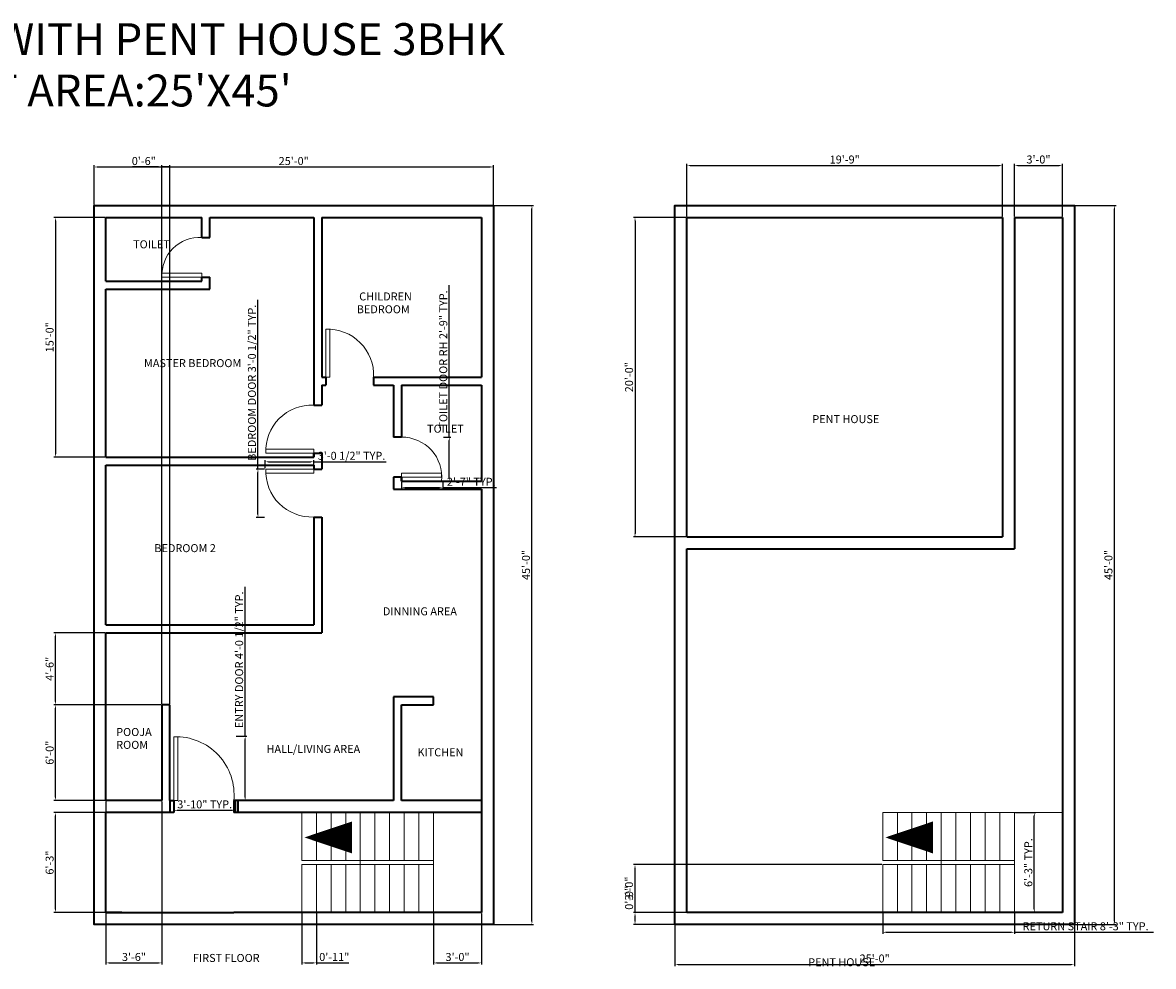
# Model space of a CAD drawing. Units: inches. Extents: x 740 to 2438, y 2555 to 3278.
# Tile 3 of 3: x 1588 to 2438, y 2570 to 3278. Entities that reach past the tile are written whole.
import ezdxf

# ---------------------------------------------------------------- set-up
doc = ezdxf.new("R2010")
doc.units = ezdxf.units.IN
doc.linetypes.add('ACAD_ISO02W100', pattern=[15, 12, -3])
for name, color, linetype, lineweight in [('A-ANNO-DIMS', 2, 'Continuous', 18), ('A-ANNO-TEXT', 7, 'Continuous', 18), ('A-AREA-IDEN', 7, 'Continuous', 18), ('A-DOOR', 3, 'Continuous', 18), ('A-FLOR-STRS', 7, 'Continuous', 18), ('A-FLOR-STRS-PATH', 2, 'ACAD_ISO02W100', 13), ('A-WALL', 7, 'Continuous', 35)]:
    doc.layers.add(name, color=color, linetype=linetype, lineweight=lineweight)
doc.styles.get("Standard").update_dxf_attribs({"font": 'arial.ttf'})
doc.dimstyles.new('ISO-25', dxfattribs={"dimtxt": 6, "dimasz": 2.5, "dimexe": 1.25, "dimexo": 0.625, "dimtad": 1, "dimdec": 1, "dimlunit": 3, "dimtxsty": 'Standard', "dimcen": 2.5, "dimadec": 0, "dimazin": 0, "dimtfac": 1, "dimtdec": 1, "dimtmove": 0, "dimatfit": 3, "dimfxl": 1, "dimarcsym": 0})

# ---------------------------------------------------------------- blocks, each defined once
blk = doc.blocks.new('DOOR-PLAN-48')
blk.add_lwpolyline([(0, 0), (3, 0), (3, 48), (0, 48)], close=True)
blk.add_arc((1.5, 4.3125), 43.7132, 354.3383149, 91.9664646)
blk = doc.blocks.new('DOOR-PLAN-36')
blk.add_lwpolyline([(36, 36), (0, 36), (0, 33), (36, 33)], close=True)
blk.add_arc((34.5, 34.5), 34.53, 177.51045, 272.48955)
blk = doc.blocks.new('DOOR-PLAN-30-L')
blk.add_lwpolyline([(30, 0), (0, 0), (0, 3), (30, 3)], close=True)
blk.add_arc((28.5, 1.5), 28.54, 86.98721, 183.01279)
blk = doc.blocks.new('DOOR-PLAN-30-R')
blk.add_lwpolyline([(0, 3), (30, 3), (30, 6), (0, 6)], close=True)
blk.add_arc((0.15, 3), 30, 354.2609, 90.28648)
blk = doc.blocks.new('STAIR-PLAN-RETURN')
for p, q in [((0, 75), (0, 39)), ((11, 75), (11, 39)), ((22, 75), (22, 39)), ((33, 75), (33, 39)), ((44, 75), (44, 0)), ((55, 75), (55, 39)), ((66, 75), (66, 39)), ((77, 75), (77, 39)), ((88, 75), (88, 39)), ((99, 75), (99, 0)), ((0, 39), (99, 39)), ((0, 36), (99, 36)), ((0, 36), (0, 0)), ((11, 36), (11, 0)), ((22, 36), (22, 0)), ((33, 36), (33, 0)), ((55, 36), (55, 0)), ((66, 36), (66, 0)), ((77, 36), (77, 0)), ((88, 36), (88, 0))]:
    blk.add_line(p, q)
blk = doc.blocks.new('STAIR-PATH-RETURN')
for points in [[(15.6, 0, 0, 0, 0), (114.75, 0, 0, 0, 0), (114.75, 41.58, 0, 0, 0), (35.71, 41.58, 96, 0, 0)], [(35.71, 41.58, 24, 0, 0), (0, 41.58, 0, 0, 0)]]:
    blk.add_lwpolyline(points, format="xyseb")
blk = doc.blocks.new('*D22')
at = {"layer": 'A-ANNO-DIMS', "color": 0, "lineweight": -2, "transparency": 16777216}
for p, q in [((2234.34, 2609.59), (2234.34, 2594.11)), ((2333.34, 2609.59), (2333.34, 2594.11)), ((2236.84, 2595.36), (2330.84, 2595.36)), ((2333.34, 2595.36), (2437.62, 2595.36))]:
    blk.add_line(p, q, dxfattribs=at)
at = {"layer": 'A-ANNO-DIMS', "color": 0, "transparency": 16777216}
for points in [[(2236.84, 2595.78), (2236.84, 2594.95), (2234.34, 2595.36)], [(2330.84, 2595.78), (2330.84, 2594.95), (2333.34, 2595.36)]]:
    blk.add_solid(points, dxfattribs=at)
at = {"layer": 'Defpoints', "color": 0, "transparency": 16777216}
for p in [(2234.34, 2610.21), (2333.34, 2610.21), (2333.34, 2595.36)]:
    blk.add_point(p, dxfattribs=at)
at = {"layer": 'A-ANNO-DIMS', "color": 0, "transparency": 16777216, "insert": (2386.73, 2599.09), "char_height": 6, "attachment_point": 5}
blk.add_mtext('RETURN STAIR 8\'-3" TYP.', dxfattribs=at)
blk = doc.blocks.new('*D23')
at = {"layer": 'A-ANNO-DIMS', "color": 0, "lineweight": -2, "transparency": 16777216}
for p, q in [((2333.97, 2685.21), (2349.44, 2685.21)), ((2348.19, 2612.71), (2348.19, 2682.71)), ((2333.97, 2610.21), (2349.44, 2610.21))]:
    blk.add_line(p, q, dxfattribs=at)
at = {"layer": 'A-ANNO-DIMS', "color": 0, "transparency": 16777216}
for points in [[(2347.78, 2682.71), (2348.61, 2682.71), (2348.19, 2685.21)], [(2347.78, 2612.71), (2348.61, 2612.71), (2348.19, 2610.21)]]:
    blk.add_solid(points, dxfattribs=at)
at = {"layer": 'Defpoints', "color": 0, "transparency": 16777216}
for p in [(2333.34, 2685.21), (2348.19, 2685.21), (2333.34, 2610.21)]:
    blk.add_point(p, dxfattribs=at)
at = {"layer": 'A-ANNO-DIMS', "color": 0, "transparency": 16777216, "insert": (2344.5, 2647.71), "char_height": 6, "attachment_point": 5, "rotation": 90}
blk.add_mtext('6\'-3" TYP.', dxfattribs=at)
blk = doc.blocks.new('*D24')
at = {"layer": 'A-ANNO-DIMS', "color": 0, "lineweight": -2, "transparency": 16777216}
for p, q in [((1765.18, 2943.21), (1765.18, 3070.36)), ((1770.02, 2943.21), (1763.93, 2943.21)), ((1765.18, 2909.29), (1765.18, 2940.71)), ((1770.02, 2906.79), (1763.93, 2906.79))]:
    blk.add_line(p, q, dxfattribs=at)
at = {"layer": 'A-ANNO-DIMS', "color": 0, "transparency": 16777216}
for points in [[(1764.77, 2940.71), (1765.6, 2940.71), (1765.18, 2943.21)], [(1764.77, 2909.29), (1765.6, 2909.29), (1765.18, 2906.79)]]:
    blk.add_solid(points, dxfattribs=at)
at = {"layer": 'Defpoints', "color": 0, "transparency": 16777216}
for p in [(1765.18, 2943.21), (1770.65, 2943.21), (1770.65, 2906.79)]:
    blk.add_point(p, dxfattribs=at)
at = {"layer": 'A-ANNO-DIMS', "color": 0, "transparency": 16777216, "insert": (1761.45, 3008.04), "char_height": 6, "attachment_point": 5, "rotation": 90}
blk.add_mtext('BEDROOM DOOR 3\'-0 1/2" TYP.', dxfattribs=at)
blk = doc.blocks.new('*D25')
at = {"layer": 'A-ANNO-DIMS', "color": 0, "lineweight": -2, "transparency": 16777216}
for p, q in [((1770.65, 2943.84), (1770.65, 2949.93)), ((1773.15, 2948.68), (1804.57, 2948.68)), ((1807.07, 2943.84), (1807.07, 2949.93)), ((1807.07, 2948.68), (1861.37, 2948.68))]:
    blk.add_line(p, q, dxfattribs=at)
at = {"layer": 'A-ANNO-DIMS', "color": 0, "transparency": 16777216}
for points in [[(1773.15, 2949.09), (1773.15, 2948.26), (1770.65, 2948.68)], [(1804.57, 2949.09), (1804.57, 2948.26), (1807.07, 2948.68)]]:
    blk.add_solid(points, dxfattribs=at)
at = {"layer": 'Defpoints', "color": 0, "transparency": 16777216}
for p in [(1807.07, 2948.68), (1770.65, 2943.21), (1807.07, 2943.21)]:
    blk.add_point(p, dxfattribs=at)
at = {"layer": 'A-ANNO-DIMS', "color": 0, "transparency": 16777216, "insert": (1835.47, 2952.41), "char_height": 6, "attachment_point": 5}
blk.add_mtext('3\'-0 1/2" TYP.', dxfattribs=at)
blk = doc.blocks.new('*D26')
at = {"layer": 'A-ANNO-DIMS', "color": 0, "lineweight": -2, "transparency": 16777216}
for p, q in [((1755.58, 2742.65), (1755.58, 2854.85)), ((1748.94, 2742.65), (1756.83, 2742.65)), ((1755.58, 2696.71), (1755.58, 2740.15)), ((1748.94, 2694.21), (1756.83, 2694.21))]:
    blk.add_line(p, q, dxfattribs=at)
at = {"layer": 'A-ANNO-DIMS', "color": 0, "transparency": 16777216}
for points in [[(1755.16, 2740.15), (1755.99, 2740.15), (1755.58, 2742.65)], [(1755.16, 2696.71), (1755.99, 2696.71), (1755.58, 2694.21)]]:
    blk.add_solid(points, dxfattribs=at)
at = {"layer": 'Defpoints', "color": 0, "transparency": 16777216}
for p in [(1748.31, 2742.65), (1755.58, 2742.65), (1748.31, 2694.21)]:
    blk.add_point(p, dxfattribs=at)
at = {"layer": 'A-ANNO-DIMS', "color": 0, "transparency": 16777216, "insert": (1751.85, 2800), "char_height": 6, "attachment_point": 5, "rotation": 90}
blk.add_mtext('ENTRY DOOR 4\'-0 1/2" TYP.', dxfattribs=at)
blk = doc.blocks.new('*D27')
at = {"layer": 'A-ANNO-DIMS', "color": 0, "lineweight": -2, "transparency": 16777216}
for p, q in [((1702.07, 2693.59), (1702.07, 2685.7)), ((1748.31, 2693.59), (1748.31, 2685.7)), ((1704.57, 2686.95), (1745.81, 2686.95))]:
    blk.add_line(p, q, dxfattribs=at)
at = {"layer": 'A-ANNO-DIMS', "color": 0, "transparency": 16777216}
for points in [[(1704.57, 2687.36), (1704.57, 2686.53), (1702.07, 2686.95)], [(1745.81, 2687.36), (1745.81, 2686.53), (1748.31, 2686.95)]]:
    blk.add_solid(points, dxfattribs=at)
at = {"layer": 'Defpoints', "color": 0, "transparency": 16777216}
for p in [(1702.07, 2694.21), (1748.31, 2694.21), (1748.31, 2686.95)]:
    blk.add_point(p, dxfattribs=at)
at = {"layer": 'A-ANNO-DIMS', "color": 0, "transparency": 16777216, "insert": (1725.19, 2690.64), "char_height": 6, "attachment_point": 5}
blk.add_mtext('3\'-10" TYP.', dxfattribs=at)
blk = doc.blocks.new('*D30')
at = {"layer": 'A-ANNO-DIMS', "color": 0, "lineweight": -2, "transparency": 16777216}
for p, q in [((1908.87, 2967.26), (1908.87, 3081.31)), ((1904.54, 2967.26), (1910.12, 2967.26)), ((1908.87, 2936.71), (1908.87, 2964.76)), ((1904.54, 2934.21), (1910.12, 2934.21))]:
    blk.add_line(p, q, dxfattribs=at)
at = {"layer": 'A-ANNO-DIMS', "color": 0, "transparency": 16777216}
for points in [[(1908.46, 2964.76), (1909.29, 2964.76), (1908.87, 2967.26)], [(1908.46, 2936.71), (1909.29, 2936.71), (1908.87, 2934.21)]]:
    blk.add_solid(points, dxfattribs=at)
at = {"layer": 'Defpoints', "color": 0, "transparency": 16777216}
for p in [(1903.92, 2967.26), (1908.87, 2967.26), (1903.92, 2934.21)]:
    blk.add_point(p, dxfattribs=at)
at = {"layer": 'A-ANNO-DIMS', "color": 0, "transparency": 16777216, "insert": (1905.15, 3025.53), "char_height": 6, "attachment_point": 5, "rotation": 90}
blk.add_mtext('TOILET DOOR RH 2\'-9" TYP.', dxfattribs=at)
blk = doc.blocks.new('*D31')
at = {"layer": 'A-ANNO-DIMS', "color": 0, "lineweight": -2, "transparency": 16777216}
for p, q in [((1873.07, 2933.59), (1873.07, 2928.01)), ((1903.92, 2933.59), (1903.92, 2928.01)), ((1875.57, 2929.26), (1901.42, 2929.26)), ((1903.92, 2929.26), (1944.34, 2929.26))]:
    blk.add_line(p, q, dxfattribs=at)
at = {"layer": 'A-ANNO-DIMS', "color": 0, "transparency": 16777216}
for points in [[(1875.57, 2929.67), (1875.57, 2928.84), (1873.07, 2929.26)], [(1901.42, 2929.67), (1901.42, 2928.84), (1903.92, 2929.26)]]:
    blk.add_solid(points, dxfattribs=at)
at = {"layer": 'Defpoints', "color": 0, "transparency": 16777216}
for p in [(1873.07, 2934.21), (1903.92, 2934.21), (1903.92, 2929.26)]:
    blk.add_point(p, dxfattribs=at)
at = {"layer": 'A-ANNO-DIMS', "color": 0, "transparency": 16777216, "insert": (1925.38, 2932.9), "char_height": 6, "attachment_point": 5}
blk.add_mtext('2\'-7" TYP.', dxfattribs=at)
blk = doc.blocks.new('*D34')
at = {"layer": 'A-ANNO-DIMS', "color": 0, "lineweight": -2, "transparency": 16777216}
for p, q in [((1642.07, 3141.84), (1642.07, 3171.31)), ((1644.57, 3170.06), (1939.57, 3170.06)), ((1942.07, 3141.84), (1942.07, 3171.31))]:
    blk.add_line(p, q, dxfattribs=at)
at = {"layer": 'A-ANNO-DIMS', "color": 0, "transparency": 16777216}
for points in [[(1644.57, 3170.48), (1644.57, 3169.65), (1642.07, 3170.06)], [(1939.57, 3170.48), (1939.57, 3169.65), (1942.07, 3170.06)]]:
    blk.add_solid(points, dxfattribs=at)
at = {"layer": 'Defpoints', "color": 0, "transparency": 16777216}
for p in [(1942.07, 3170.06), (1642.07, 3141.21), (1942.07, 3141.21)]:
    blk.add_point(p, dxfattribs=at)
at = {"layer": 'A-ANNO-DIMS', "color": 0, "transparency": 16777216, "insert": (1792.07, 3173.75), "char_height": 6, "attachment_point": 5}
blk.add_mtext('25\'-0"', dxfattribs=at)
blk = doc.blocks.new('*D35')
at = {"layer": 'A-ANNO-DIMS', "color": 0, "lineweight": -2, "transparency": 16777216}
for p, q in [((1942.69, 3141.21), (1972.17, 3141.21)), ((1970.92, 2603.71), (1970.92, 3138.71)), ((1942.69, 2601.21), (1972.17, 2601.21))]:
    blk.add_line(p, q, dxfattribs=at)
at = {"layer": 'A-ANNO-DIMS', "color": 0, "transparency": 16777216}
for points in [[(1970.5, 3138.71), (1971.33, 3138.71), (1970.92, 3141.21)], [(1970.5, 2603.71), (1971.33, 2603.71), (1970.92, 2601.21)]]:
    blk.add_solid(points, dxfattribs=at)
at = {"layer": 'Defpoints', "color": 0, "transparency": 16777216}
for p in [(1942.07, 3141.21), (1970.92, 3141.21), (1942.07, 2601.21)]:
    blk.add_point(p, dxfattribs=at)
at = {"layer": 'A-ANNO-DIMS', "color": 0, "transparency": 16777216, "insert": (1967.23, 2871.21), "char_height": 6, "attachment_point": 5, "rotation": 90}
blk.add_mtext('45\'-0"', dxfattribs=at)
blk = doc.blocks.new('*D36')
at = {"layer": 'A-ANNO-DIMS', "color": 0, "lineweight": -2, "transparency": 16777216}
for p, q in [((2078.34, 2600.59), (2078.34, 2569.96)), ((2378.34, 2600.59), (2378.34, 2569.96)), ((2080.84, 2571.21), (2375.84, 2571.21))]:
    blk.add_line(p, q, dxfattribs=at)
at = {"layer": 'A-ANNO-DIMS', "color": 0, "transparency": 16777216}
for points in [[(2080.84, 2571.63), (2080.84, 2570.8), (2078.34, 2571.21)], [(2375.84, 2571.63), (2375.84, 2570.8), (2378.34, 2571.21)]]:
    blk.add_solid(points, dxfattribs=at)
at = {"layer": 'Defpoints', "color": 0, "transparency": 16777216}
for p in [(2078.34, 2601.21), (2378.34, 2601.21), (2378.34, 2571.21)]:
    blk.add_point(p, dxfattribs=at)
at = {"layer": 'A-ANNO-DIMS', "color": 0, "transparency": 16777216, "insert": (2228.34, 2574.9), "char_height": 6, "attachment_point": 5}
blk.add_mtext('25\'-0"', dxfattribs=at)
blk = doc.blocks.new('*D37')
at = {"layer": 'A-ANNO-DIMS', "color": 0, "lineweight": -2, "transparency": 16777216}
for p, q in [((2378.97, 3141.21), (2409.59, 3141.21)), ((2408.34, 2603.71), (2408.34, 3138.71)), ((2378.97, 2601.21), (2409.59, 2601.21))]:
    blk.add_line(p, q, dxfattribs=at)
at = {"layer": 'A-ANNO-DIMS', "color": 0, "transparency": 16777216}
for points in [[(2407.93, 3138.71), (2408.76, 3138.71), (2408.34, 3141.21)], [(2407.93, 2603.71), (2408.76, 2603.71), (2408.34, 2601.21)]]:
    blk.add_solid(points, dxfattribs=at)
at = {"layer": 'Defpoints', "color": 0, "transparency": 16777216}
for p in [(2378.34, 3141.21), (2408.34, 3141.21), (2378.34, 2601.21)]:
    blk.add_point(p, dxfattribs=at)
at = {"layer": 'A-ANNO-DIMS', "color": 0, "transparency": 16777216, "insert": (2404.66, 2871.21), "char_height": 6, "attachment_point": 5, "rotation": 90}
blk.add_mtext('45\'-0"', dxfattribs=at)
blk = doc.blocks.new('*D38')
at = {"layer": 'A-ANNO-DIMS', "color": 0, "lineweight": -2, "transparency": 16777216}
for p, q in [((2087.34, 3132.84), (2087.34, 3172.46)), ((2089.84, 3171.21), (2321.84, 3171.21)), ((2324.34, 3132.84), (2324.34, 3172.46))]:
    blk.add_line(p, q, dxfattribs=at)
at = {"layer": 'A-ANNO-DIMS', "color": 0, "transparency": 16777216}
for points in [[(2089.84, 3171.63), (2089.84, 3170.8), (2087.34, 3171.21)], [(2321.84, 3171.63), (2321.84, 3170.8), (2324.34, 3171.21)]]:
    blk.add_solid(points, dxfattribs=at)
at = {"layer": 'Defpoints', "color": 0, "transparency": 16777216}
for p in [(2324.34, 3171.21), (2087.34, 3132.21), (2324.34, 3132.21)]:
    blk.add_point(p, dxfattribs=at)
at = {"layer": 'A-ANNO-DIMS', "color": 0, "transparency": 16777216, "insert": (2205.84, 3174.9), "char_height": 6, "attachment_point": 5}
blk.add_mtext('19\'-9"', dxfattribs=at)
blk = doc.blocks.new('*D39')
at = {"layer": 'A-ANNO-DIMS', "color": 0, "lineweight": -2, "transparency": 16777216}
for p, q in [((2086.72, 3132.21), (2047.09, 3132.21)), ((2048.34, 3129.71), (2048.34, 2894.71)), ((2086.72, 2892.21), (2047.09, 2892.21))]:
    blk.add_line(p, q, dxfattribs=at)
at = {"layer": 'A-ANNO-DIMS', "color": 0, "transparency": 16777216}
for points in [[(2047.93, 3129.71), (2048.76, 3129.71), (2048.34, 3132.21)], [(2047.93, 2894.71), (2048.76, 2894.71), (2048.34, 2892.21)]]:
    blk.add_solid(points, dxfattribs=at)
at = {"layer": 'Defpoints', "color": 0, "transparency": 16777216}
for p in [(2087.34, 3132.21), (2048.34, 2892.21), (2087.34, 2892.21)]:
    blk.add_point(p, dxfattribs=at)
at = {"layer": 'A-ANNO-DIMS', "color": 0, "transparency": 16777216, "insert": (2044.66, 3012.21), "char_height": 6, "attachment_point": 5, "rotation": 90}
blk.add_mtext('20\'-0"', dxfattribs=at)
blk = doc.blocks.new('*D40')
at = {"layer": 'A-ANNO-DIMS', "color": 0, "lineweight": -2, "transparency": 16777216}
for p, q in [((2333.34, 3132.84), (2333.34, 3172.46)), ((2335.84, 3171.21), (2366.84, 3171.21)), ((2369.34, 3132.84), (2369.34, 3172.46))]:
    blk.add_line(p, q, dxfattribs=at)
at = {"layer": 'A-ANNO-DIMS', "color": 0, "transparency": 16777216}
for points in [[(2335.84, 3171.63), (2335.84, 3170.8), (2333.34, 3171.21)], [(2366.84, 3171.63), (2366.84, 3170.8), (2369.34, 3171.21)]]:
    blk.add_solid(points, dxfattribs=at)
at = {"layer": 'Defpoints', "color": 0, "transparency": 16777216}
for p in [(2369.34, 3171.21), (2333.34, 3132.21), (2369.34, 3132.21)]:
    blk.add_point(p, dxfattribs=at)
at = {"layer": 'A-ANNO-DIMS', "color": 0, "transparency": 16777216, "insert": (2351.34, 3174.9), "char_height": 6, "attachment_point": 5}
blk.add_mtext('3\'-0"', dxfattribs=at)
blk = doc.blocks.new('*D41')
at = {"layer": 'A-ANNO-DIMS', "color": 0, "lineweight": -2, "transparency": 16777216}
for p, q in [((2048.34, 2610.21), (2048.34, 2629.91)), ((2086.72, 2610.21), (2047.09, 2610.21)), ((2048.34, 2603.71), (2048.34, 2607.71)), ((2077.72, 2601.21), (2047.09, 2601.21))]:
    blk.add_line(p, q, dxfattribs=at)
at = {"layer": 'A-ANNO-DIMS', "color": 0, "transparency": 16777216}
for points in [[(2047.93, 2607.71), (2048.76, 2607.71), (2048.34, 2610.21)], [(2047.93, 2603.71), (2048.76, 2603.71), (2048.34, 2601.21)]]:
    blk.add_solid(points, dxfattribs=at)
at = {"layer": 'Defpoints', "color": 0, "transparency": 16777216}
for p in [(2048.34, 2610.21), (2087.34, 2610.21), (2078.34, 2601.21)]:
    blk.add_point(p, dxfattribs=at)
at = {"layer": 'A-ANNO-DIMS', "color": 0, "transparency": 16777216, "insert": (2044.66, 2621.31), "char_height": 6, "attachment_point": 5, "rotation": 90}
blk.add_mtext('0\'-9"', dxfattribs=at)
blk = doc.blocks.new('*D42')
at = {"layer": 'A-ANNO-DIMS', "color": 0, "lineweight": -2, "transparency": 16777216}
for p, q in [((2233.72, 2646.21), (2047.09, 2646.21)), ((2048.34, 2612.71), (2048.34, 2643.71)), ((2233.72, 2610.21), (2047.09, 2610.21))]:
    blk.add_line(p, q, dxfattribs=at)
at = {"layer": 'A-ANNO-DIMS', "color": 0, "transparency": 16777216}
for points in [[(2047.93, 2643.71), (2048.76, 2643.71), (2048.34, 2646.21)], [(2047.93, 2612.71), (2048.76, 2612.71), (2048.34, 2610.21)]]:
    blk.add_solid(points, dxfattribs=at)
at = {"layer": 'Defpoints', "color": 0, "transparency": 16777216}
for p in [(2048.34, 2646.21), (2234.34, 2646.21), (2234.34, 2610.21)]:
    blk.add_point(p, dxfattribs=at)
at = {"layer": 'A-ANNO-DIMS', "color": 0, "transparency": 16777216, "insert": (2044.65, 2628.21), "char_height": 6, "attachment_point": 5, "rotation": 90}
blk.add_mtext('3\'-0"', dxfattribs=at)
blk = doc.blocks.new('*D43')
at = {"layer": 'A-ANNO-DIMS', "color": 0, "lineweight": -2, "transparency": 16777216}
for p, q in [((1798.07, 2609.59), (1798.07, 2571.11)), ((1809.07, 2609.59), (1809.07, 2571.11)), ((1800.57, 2572.36), (1806.57, 2572.36)), ((1809.07, 2572.36), (1833.43, 2572.36))]:
    blk.add_line(p, q, dxfattribs=at)
at = {"layer": 'A-ANNO-DIMS', "color": 0, "transparency": 16777216}
for points in [[(1800.57, 2572.78), (1800.57, 2571.95), (1798.07, 2572.36)], [(1806.57, 2572.78), (1806.57, 2571.95), (1809.07, 2572.36)]]:
    blk.add_solid(points, dxfattribs=at)
at = {"layer": 'Defpoints', "color": 0, "transparency": 16777216}
for p in [(1798.07, 2610.21), (1809.07, 2610.21), (1809.07, 2572.36)]:
    blk.add_point(p, dxfattribs=at)
at = {"layer": 'A-ANNO-DIMS', "color": 0, "transparency": 16777216, "insert": (1822.5, 2576.05), "char_height": 6, "attachment_point": 5}
blk.add_mtext('0\'-11"', dxfattribs=at)
blk = doc.blocks.new('*D44')
at = {"layer": 'A-ANNO-DIMS', "color": 0, "lineweight": -2, "transparency": 16777216}
for p, q in [((1897.07, 2609.59), (1897.07, 2571.11)), ((1933.07, 2609.59), (1933.07, 2571.11)), ((1899.57, 2572.36), (1930.57, 2572.36))]:
    blk.add_line(p, q, dxfattribs=at)
at = {"layer": 'A-ANNO-DIMS', "color": 0, "transparency": 16777216}
for points in [[(1899.57, 2572.78), (1899.57, 2571.95), (1897.07, 2572.36)], [(1930.57, 2572.78), (1930.57, 2571.95), (1933.07, 2572.36)]]:
    blk.add_solid(points, dxfattribs=at)
at = {"layer": 'Defpoints', "color": 0, "transparency": 16777216}
for p in [(1897.07, 2610.21), (1933.07, 2610.21), (1933.07, 2572.36)]:
    blk.add_point(p, dxfattribs=at)
at = {"layer": 'A-ANNO-DIMS', "color": 0, "transparency": 16777216, "insert": (1915.07, 2576.05), "char_height": 6, "attachment_point": 5}
blk.add_mtext('3\'-0"', dxfattribs=at)
blk = doc.blocks.new('*D71')
at = {"layer": 'A-ANNO-DIMS', "color": 0, "lineweight": -2, "transparency": 16777216}
for p, q in [((1651.07, 2693.59), (1651.07, 2571.11)), ((1693.07, 2693.59), (1693.07, 2571.11)), ((1653.57, 2572.36), (1690.57, 2572.36))]:
    blk.add_line(p, q, dxfattribs=at)
at = {"layer": 'A-ANNO-DIMS', "color": 0, "transparency": 16777216}
for points in [[(1653.57, 2572.78), (1653.57, 2571.95), (1651.07, 2572.36)], [(1690.57, 2572.78), (1690.57, 2571.95), (1693.07, 2572.36)]]:
    blk.add_solid(points, dxfattribs=at)
at = {"layer": 'Defpoints', "color": 0, "transparency": 16777216}
for p in [(1651.07, 2694.21), (1693.07, 2694.21), (1693.07, 2572.36)]:
    blk.add_point(p, dxfattribs=at)
at = {"layer": 'A-ANNO-DIMS', "color": 0, "transparency": 16777216, "insert": (1672.07, 2576.05), "char_height": 6, "attachment_point": 5}
blk.add_mtext('3\'-6"', dxfattribs=at)
blk = doc.blocks.new('*D72')
at = {"layer": 'A-ANNO-DIMS', "color": 0, "lineweight": -2, "transparency": 16777216}
for p, q in [((1692.44, 2766.21), (1611.97, 2766.21)), ((1613.22, 2696.71), (1613.22, 2763.71)), ((1692.44, 2694.21), (1611.97, 2694.21))]:
    blk.add_line(p, q, dxfattribs=at)
at = {"layer": 'A-ANNO-DIMS', "color": 0, "transparency": 16777216}
for points in [[(1612.8, 2763.71), (1613.63, 2763.71), (1613.22, 2766.21)], [(1612.8, 2696.71), (1613.63, 2696.71), (1613.22, 2694.21)]]:
    blk.add_solid(points, dxfattribs=at)
at = {"layer": 'Defpoints', "color": 0, "transparency": 16777216}
for p in [(1613.22, 2766.21), (1693.07, 2766.21), (1693.07, 2694.21)]:
    blk.add_point(p, dxfattribs=at)
at = {"layer": 'A-ANNO-DIMS', "color": 0, "transparency": 16777216, "insert": (1609.53, 2730.21), "char_height": 6, "attachment_point": 5, "rotation": 90}
blk.add_mtext('6\'-0"', dxfattribs=at)
blk = doc.blocks.new('*D73')
at = {"layer": 'A-ANNO-DIMS', "color": 0, "lineweight": -2, "transparency": 16777216}
for p, q in [((1650.44, 2820.21), (1611.97, 2820.21)), ((1613.22, 2768.71), (1613.22, 2817.71)), ((1692.44, 2766.21), (1611.97, 2766.21))]:
    blk.add_line(p, q, dxfattribs=at)
at = {"layer": 'A-ANNO-DIMS', "color": 0, "transparency": 16777216}
for points in [[(1612.8, 2817.71), (1613.63, 2817.71), (1613.22, 2820.21)], [(1612.8, 2768.71), (1613.63, 2768.71), (1613.22, 2766.21)]]:
    blk.add_solid(points, dxfattribs=at)
at = {"layer": 'Defpoints', "color": 0, "transparency": 16777216}
for p in [(1613.22, 2820.21), (1651.07, 2820.21), (1693.07, 2766.21)]:
    blk.add_point(p, dxfattribs=at)
at = {"layer": 'A-ANNO-DIMS', "color": 0, "transparency": 16777216, "insert": (1609.53, 2793.21), "char_height": 6, "attachment_point": 5, "rotation": 90}
blk.add_mtext('4\'-6"', dxfattribs=at)
blk = doc.blocks.new('*D74')
at = {"layer": 'A-ANNO-DIMS', "color": 0, "lineweight": -2, "transparency": 16777216}
for p, q in [((1650.44, 2685.21), (1611.97, 2685.21)), ((1613.22, 2612.71), (1613.22, 2682.71)), ((1650.44, 2610.21), (1611.97, 2610.21))]:
    blk.add_line(p, q, dxfattribs=at)
at = {"layer": 'A-ANNO-DIMS', "color": 0, "transparency": 16777216}
for points in [[(1612.8, 2682.71), (1613.63, 2682.71), (1613.22, 2685.21)], [(1612.8, 2612.71), (1613.63, 2612.71), (1613.22, 2610.21)]]:
    blk.add_solid(points, dxfattribs=at)
at = {"layer": 'Defpoints', "color": 0, "transparency": 16777216}
for p in [(1613.22, 2685.21), (1651.07, 2685.21), (1651.07, 2610.21)]:
    blk.add_point(p, dxfattribs=at)
at = {"layer": 'A-ANNO-DIMS', "color": 0, "transparency": 16777216, "insert": (1609.53, 2647.71), "char_height": 6, "attachment_point": 5, "rotation": 90}
blk.add_mtext('6\'-3"', dxfattribs=at)
blk = doc.blocks.new('*D75')
at = {"layer": 'A-ANNO-DIMS', "color": 0, "lineweight": -2, "transparency": 16777216}
for p, q in [((1650.44, 3132.21), (1611.97, 3132.21)), ((1613.22, 3129.71), (1613.22, 2954.71)), ((1650.44, 2952.21), (1611.97, 2952.21))]:
    blk.add_line(p, q, dxfattribs=at)
at = {"layer": 'A-ANNO-DIMS', "color": 0, "transparency": 16777216}
for points in [[(1612.8, 3129.71), (1613.63, 3129.71), (1613.22, 3132.21)], [(1612.8, 2954.71), (1613.63, 2954.71), (1613.22, 2952.21)]]:
    blk.add_solid(points, dxfattribs=at)
at = {"layer": 'Defpoints', "color": 0, "transparency": 16777216}
for p in [(1651.07, 3132.21), (1613.22, 2952.21), (1651.07, 2952.21)]:
    blk.add_point(p, dxfattribs=at)
at = {"layer": 'A-ANNO-DIMS', "color": 0, "transparency": 16777216, "insert": (1609.53, 3042.21), "char_height": 6, "attachment_point": 5, "rotation": 90}
blk.add_mtext('15\'-0"', dxfattribs=at)
blk = doc.blocks.new('*D78')
at = {"layer": 'A-ANNO-DIMS', "color": 0, "lineweight": -2, "transparency": 16777216}
for p, q in [((1690.57, 3170.06), (1670.87, 3170.06)), ((1693.07, 2766.84), (1693.07, 3171.31)), ((1699.07, 3170.06), (1693.07, 3170.06)), ((1699.07, 2766.84), (1699.07, 3171.31)), ((1701.57, 3170.06), (1704.07, 3170.06))]:
    blk.add_line(p, q, dxfattribs=at)
at = {"layer": 'A-ANNO-DIMS', "color": 0, "transparency": 16777216}
for points in [[(1690.57, 3170.48), (1690.57, 3169.65), (1693.07, 3170.06)], [(1701.57, 3170.48), (1701.57, 3169.65), (1699.07, 3170.06)]]:
    blk.add_solid(points, dxfattribs=at)
at = {"layer": 'Defpoints', "color": 0, "transparency": 16777216}
for p in [(1693.07, 3170.06), (1693.07, 2766.21), (1699.07, 2766.21)]:
    blk.add_point(p, dxfattribs=at)
at = {"layer": 'A-ANNO-DIMS', "color": 0, "transparency": 16777216, "insert": (1679.47, 3173.75), "char_height": 6, "attachment_point": 5}
blk.add_mtext('0\'-6"', dxfattribs=at)

msp = doc.modelspace()

# ---------------------------------------------------------------- linework, layer by layer
at = {"layer": 'A-FLOR-STRS'}
msp.add_line((2234.34, 2685.21), (2369.34, 2685.21), dxfattribs=at)
at = {"layer": 'A-WALL'}
for p, q in [((1651.07, 3132.21), (1723.07, 3132.21)), ((1651.07, 3084.21), (1651.07, 3132.21)), ((1723.07, 3117.21), (1723.07, 3132.21)), ((1729.07, 3132.21), (1807.07, 3132.21)), ((1729.07, 3117.21), (1729.07, 3132.21)), ((1807.07, 3132.21), (1807.07, 2991.21)), ((1813.07, 3132.21), (1933.07, 3132.21)), ((1813.07, 3132.21), (1813.07, 3012.21)), ((1933.07, 3132.21), (1933.07, 3012.21)), ((2087.34, 3132.21), (2324.34, 3132.21)), ((2087.34, 2892.21), (2087.34, 3132.21)), ((2324.34, 3132.21), (2324.34, 2892.21)), ((2333.34, 3132.21), (2333.34, 2883.21)), ((2333.34, 3132.21), (2369.34, 3132.21)), ((2369.34, 3132.21), (2369.34, 2883.21)), ((1723.07, 3117.21), (1729.07, 3117.21)), ((1651.07, 3084.21), (1723.07, 3084.21)), ((1723.07, 3084.21), (1723.07, 3087.21)), ((1723.07, 3084.21), (1723.07, 3087.21)), ((1723.07, 3087.21), (1729.07, 3087.21)), ((1729.07, 3078.21), (1729.07, 3087.21)), ((1651.07, 3078.21), (1729.07, 3078.21)), ((1651.07, 2952.21), (1651.07, 3078.21)), ((1813.07, 3012.21), (1816.07, 3012.21)), ((1813.07, 3012.21), (1816.07, 3012.21)), ((1813.07, 3006.21), (1816.07, 3006.21)), ((1813.07, 3006.21), (1813.07, 2991.21)), ((1816.07, 3012.21), (1816.07, 3006.21)), ((1852.07, 3012.21), (1933.07, 3012.21)), ((1852.07, 3012.21), (1852.07, 3006.21)), ((1852.07, 3006.21), (1867.07, 3006.21)), ((1867.07, 3006.21), (1867.07, 2967.21)), ((1873.07, 3006.21), (1933.07, 3006.21)), ((1873.07, 3006.21), (1873.07, 2967.21)), ((1933.07, 3006.21), (1933.07, 2934.21)), ((1807.07, 2991.21), (1813.07, 2991.21)), ((1873.07, 2967.21), (1867.07, 2967.21)), ((1807.07, 2955.21), (1807.07, 2952.21)), ((1807.07, 2952.21), (1807.07, 2955.21)), ((1807.07, 2955.21), (1813.07, 2955.21)), ((1813.07, 2955.21), (1813.07, 2943.21)), ((1651.07, 2952.21), (1807.07, 2952.21)), ((1651.07, 2946.21), (1807.07, 2946.21)), ((1651.07, 2826.21), (1651.07, 2946.21)), ((1807.07, 2946.21), (1807.07, 2943.21)), ((1807.07, 2946.21), (1807.07, 2943.21)), ((1807.07, 2943.21), (1813.07, 2943.21)), ((1867.07, 2937.21), (1867.07, 2928.21)), ((1873.07, 2937.21), (1867.07, 2937.21)), ((1873.07, 2937.21), (1873.07, 2934.21)), ((1873.07, 2934.21), (1873.07, 2937.21)), ((1873.07, 2934.21), (1933.07, 2934.21)), ((1867.07, 2928.21), (1933.07, 2928.21)), ((1933.07, 2928.21), (1933.07, 2610.21)), ((1807.07, 2907.21), (1807.07, 2826.21)), ((1807.07, 2907.21), (1813.07, 2907.21)), ((1813.07, 2907.21), (1813.07, 2820.21)), ((2087.34, 2892.21), (2324.34, 2892.21)), ((2087.34, 2610.21), (2087.34, 2883.21)), ((2087.34, 2883.21), (2333.34, 2883.21)), ((2369.34, 2883.21), (2369.34, 2610.21)), ((1651.07, 2826.21), (1807.07, 2826.21)), ((1651.07, 2820.21), (1813.07, 2820.21)), ((1651.07, 2694.21), (1651.07, 2820.21)), ((1897.07, 2772.21), (1867.07, 2772.21)), ((1867.07, 2772.21), (1867.07, 2766.21)), ((1897.07, 2766.21), (1897.07, 2772.21)), ((1699.07, 2766.21), (1693.07, 2766.21)), ((1693.07, 2766.21), (1693.07, 2694.21)), ((1699.07, 2694.21), (1699.07, 2766.21)), ((1867.07, 2766.21), (1867.07, 2694.21)), ((1873.07, 2694.21), (1873.07, 2766.21)), ((1873.07, 2766.21), (1897.07, 2766.21)), ((1693.07, 2694.21), (1651.07, 2694.21)), ((1699.07, 2694.21), (1699.07, 2685.21)), ((1699.07, 2694.21), (1702.07, 2694.21)), ((1702.07, 2694.21), (1702.07, 2685.21)), ((1867.07, 2694.21), (1747.07, 2694.21)), ((1747.07, 2694.21), (1747.07, 2685.21)), ((1750.07, 2694.21), (1750.07, 2685.21)), ((1933.07, 2694.21), (1873.07, 2694.21)), ((1699.07, 2685.21), (1651.07, 2685.21)), ((1651.07, 2610.21), (1651.07, 2685.21)), ((1702.07, 2685.21), (1699.07, 2685.21)), ((1933.07, 2685.21), (1747.07, 2685.21)), ((1663.07, 2610.21), (1651.07, 2610.21)), ((1651.07, 2610.21), (1747.07, 2610.21)), ((1933.07, 2610.21), (1747.07, 2610.21)), ((2369.34, 2610.21), (2087.34, 2610.21))]:
    msp.add_line(p, q, dxfattribs=at)
for points in [[(1747.07, 2601.21), (1642.07, 2601.21), (1642.07, 3141.21), (1942.07, 3141.21), (1942.07, 2601.21), (1747.07, 2601.21)], [(2378.34, 2601.21), (2078.34, 2601.21), (2078.34, 3141.21), (2378.34, 3141.21), (2378.34, 2601.21), (2183.34, 2601.21)]]:
    msp.add_lwpolyline(points, dxfattribs=at)

# ---------------------------------------------------------------- block references
at = {"layer": 'A-DOOR'}
for name, p in [('DOOR-PLAN-30-L', (1693.07, 3087.21)), ('DOOR-PLAN-30-R', (1873.07, 2934.21)), ('DOOR-PLAN-36', (1771.07, 2907.21)), ('DOOR-PLAN-48', (1702.07, 2694.21))]:
    msp.add_blockref(name, p, dxfattribs=at)
at = {"layer": 'A-DOOR', "extrusion": (0, 0, -1), "zscale": -1}
for p, rotation in [((-1852.07, 3048.21), 269.9999999999956), ((-1771.07, 2991.21), 180)]:
    msp.add_blockref('DOOR-PLAN-36', p, dxfattribs=dict(at, rotation=rotation))
at = {"layer": 'A-FLOR-STRS'}
for p in [(1798.07, 2610.21), (2234.34, 2610.21)]:
    msp.add_blockref('STAIR-PLAN-RETURN', p, dxfattribs=at)
at = {"layer": 'A-FLOR-STRS-PATH'}
for p in [(1800.06, 2625), (2236.34, 2625)]:
    msp.add_blockref('STAIR-PATH-RETURN', p, dxfattribs=at)

# ---------------------------------------------------------------- texts
at = {"layer": 'A-ANNO-TEXT'}
for s, height, p in [('G+1 WITH PENT HOUSE 3BHK', 24, (1502.24, 3254.05)), ("PLOT AREA:25'X45'", 24, (1502.24, 3215.5)), ('FIRST FLOOR', 6, (1716.4, 2573.08)), ('PENT HOUSE', 6, (2178.4, 2569.86))]:
    msp.add_text(s, height=height, dxfattribs=at).set_placement(p)
at = {"layer": 'A-AREA-IDEN'}
for s, p in [('TOILET', (1671.44, 3109)), (' CHILDREN ', (1839.38, 3069.85)), ('BEDROOM', (1839.38, 3060.21)), ('MASTER BEDROOM', (1679.61, 3019.77)), ('PENT HOUSE', (2181.49, 2977.71)), ('TOILET', (1892.19, 2970.53)), ('BEDROOM 2', (1687.37, 2880.83)), ('DINNING AREA', (1858.98, 2833.39)), ('POOJA ', (1658.73, 2742.75)), ('ROOM', (1658.73, 2733.11)), ('HALL/LIVING AREA', (1771.61, 2730.03)), ('KITCHEN', (1884.94, 2727.52))]:
    msp.add_text(s, height=6, dxfattribs=at).set_placement(p)

# ---------------------------------------------------------------- dimensions: what is measured, and where the dimension line sits
at = {"layer": 'A-ANNO-DIMS'}
for base, p1, p2, picture, middle in [((1942.07, 3170.06), (1642.07, 3141.21), (1942.07, 3141.21), '*D34', (1792.07, 3173.75)), ((1693.07, 3170.06), (1699.07, 2766.21), (1693.07, 2766.21), '*D78', (1679.47, 3173.75)), ((2324.34, 3171.21), (2087.34, 3132.21), (2324.34, 3132.21), '*D38', (2205.84, 3174.9)), ((2369.34, 3171.21), (2333.34, 3132.21), (2369.34, 3132.21), '*D40', (2351.34, 3174.9)), ((1693.07, 2572.36), (1651.07, 2694.21), (1693.07, 2694.21), '*D71', (1672.07, 2576.05)), ((1809.07, 2572.36), (1798.07, 2610.21), (1809.07, 2610.21), '*D43', (1822.5, 2576.05)), ((1933.07, 2572.36), (1897.07, 2610.21), (1933.07, 2610.21), '*D44', (1915.07, 2576.05)), ((2378.34, 2571.21), (2078.34, 2601.21), (2378.34, 2601.21), '*D36', (2228.34, 2574.9))]:
    dim = msp.add_linear_dim(base=base, p1=p1, p2=p2, dimstyle='ISO-25', override={"dimdec": 1, "dimlfac": 1, "dimrnd": 0, "dimzin": 1, "dimdsep": 46, "dimlunit": 4, "dimfrac": 2}, dxfattribs=at)
    dim.commit()
    dim.dimension.update_dxf_attribs({"geometry": picture, "text_midpoint": middle})
for base, p1, p2, picture, middle in [((1970.92, 3141.21), (1942.07, 2601.21), (1942.07, 3141.21), '*D35', (1967.23, 2871.21)), ((2408.34, 3141.21), (2378.34, 2601.21), (2378.34, 3141.21), '*D37', (2404.66, 2871.21)), ((1613.22, 2952.21), (1651.07, 3132.21), (1651.07, 2952.21), '*D75', (1609.53, 3042.21)), ((2048.34, 2892.21), (2087.34, 3132.21), (2087.34, 2892.21), '*D39', (2044.66, 3012.21)), ((1613.22, 2820.21), (1693.07, 2766.21), (1651.07, 2820.21), '*D73', (1609.53, 2793.21)), ((1613.22, 2766.21), (1693.07, 2694.21), (1693.07, 2766.21), '*D72', (1609.53, 2730.21)), ((1613.22, 2685.21), (1651.07, 2610.21), (1651.07, 2685.21), '*D74', (1609.53, 2647.71)), ((2048.34, 2646.21), (2234.34, 2610.21), (2234.34, 2646.21), '*D42', (2044.65, 2628.21)), ((2048.34, 2610.21), (2078.34, 2601.21), (2087.34, 2610.21), '*D41', (2044.66, 2621.31))]:
    dim = msp.add_linear_dim(base=base, p1=p1, p2=p2, angle=90, dimstyle='ISO-25', override={"dimdec": 1, "dimlfac": 1, "dimrnd": 0, "dimzin": 1, "dimdsep": 46, "dimlunit": 4, "dimfrac": 2}, dxfattribs=at)
    dim.commit()
    dim.dimension.update_dxf_attribs({"geometry": picture, "text_midpoint": middle})
for base, p1, p2, text, picture, middle in [((1908.8747, 2967.2555), (1903.9184, 2934.213), (1903.9184, 2967.2555), 'TOILET DOOR RH <> TYP.', '*D30', (1905.1454, 3025.5326)), ((1765.18, 2943.21), (1770.65, 2906.79), (1770.65, 2943.21), 'BEDROOM DOOR <> TYP.', '*D24', (1761.45, 3008.04)), ((1755.58, 2742.65), (1748.31, 2694.21), (1748.31, 2742.65), 'ENTRY DOOR <> TYP.', '*D26', (1751.85, 2800)), ((2348.19, 2685.21), (2333.34, 2610.21), (2333.34, 2685.21), '<> TYP.', '*D23', (2344.5, 2647.71))]:
    dim = msp.add_linear_dim(base=base, p1=p1, p2=p2, angle=90, text=text, dimstyle='ISO-25', override={"dimdec": 1, "dimlfac": 1, "dimrnd": 0, "dimzin": 1, "dimdsep": 46, "dimlunit": 4, "dimfrac": 2}, dxfattribs=at)
    dim.commit()
    dim.dimension.update_dxf_attribs({"geometry": picture, "text_midpoint": middle})
for base, p1, p2, text, picture, middle in [((1807.07, 2948.68), (1770.65, 2943.21), (1807.07, 2943.21), '<> TYP.', '*D25', (1835.47, 2952.41)), ((1903.9184, 2929.2566), (1873.0679, 2934.213), (1903.9184, 2934.213), '<> TYP.', '*D31', (1925.381, 2932.8959)), ((1748.31, 2686.95), (1702.07, 2694.21), (1748.31, 2694.21), '<> TYP.', '*D27', (1725.19, 2690.64)), ((2333.34, 2595.36), (2234.34, 2610.21), (2333.34, 2610.21), 'RETURN STAIR <> TYP.', '*D22', (2386.73, 2599.09))]:
    dim = msp.add_linear_dim(base=base, p1=p1, p2=p2, text=text, dimstyle='ISO-25', override={"dimdec": 1, "dimlfac": 1, "dimrnd": 0, "dimzin": 1, "dimdsep": 46, "dimlunit": 4, "dimfrac": 2}, dxfattribs=at)
    dim.commit()
    dim.dimension.update_dxf_attribs({"geometry": picture, "text_midpoint": middle})

doc.saveas('drawing.dxf')
